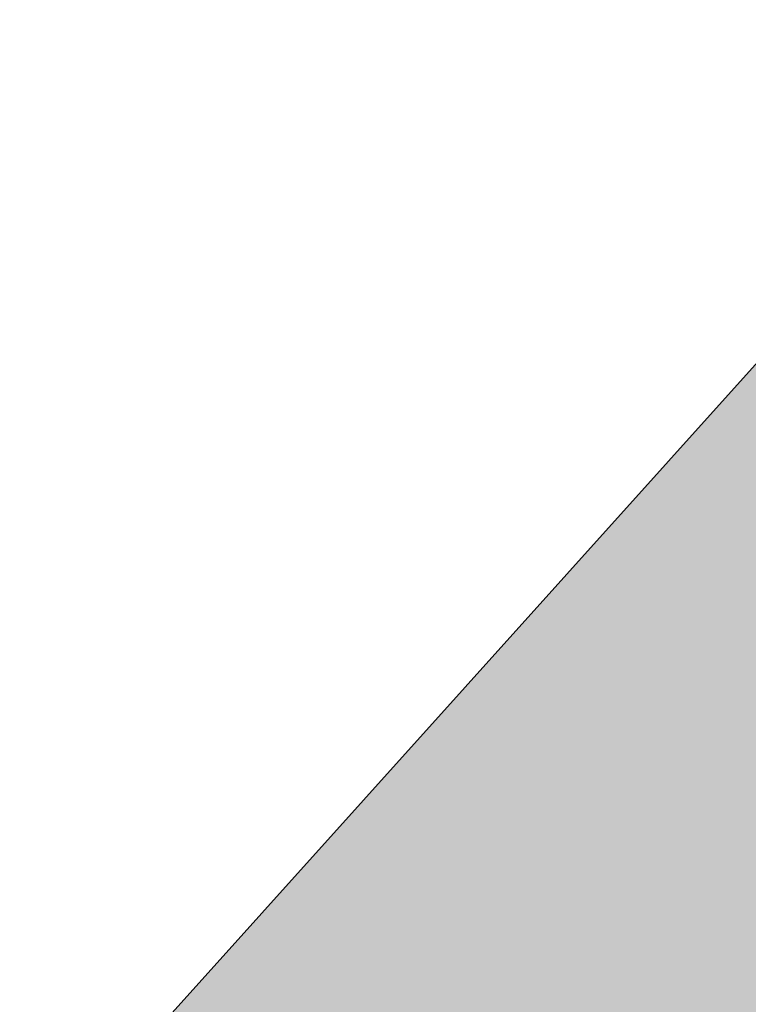
# Model space of a CAD drawing. Units: inches. Extents: x 2091 to 2899, y 967 to 2217.
# Tile 246 of 256: x 2213.354327 to 2213.360613, y 1136.678717 to 1136.687206. Entities that reach past the tile are written whole.
import ezdxf

# ---------------------------------------------------------------- set-up
doc = ezdxf.new("R2010")
doc.units = ezdxf.units.IN
doc.layers.add('L-PLNT-PATT', color=114, linetype='Continuous', lineweight=13, true_color=0x139b48)
doc.layers.add('L-PLNT-TREE', color=94, linetype='Continuous', lineweight=13)

# ---------------------------------------------------------------- blocks, each defined once
blk = doc.blocks.new('*U25')
blk.add_lwpolyline([(-1139.42368, 1783.79628), (-1216.11644, 1685.47796), (-1117.5111, 1601.2033), (-1051.7759, 1643.3419), (-1126.09884, 1521.20092), (-1072.10606, 1527.49758), (-1079.90386, 1416.93646), (-1259.93906, 1179.83508), (-1479.05978, 1165.78888), (-1577.66258, 1109.60662), (-1742.00312, 927.01364), (-1676.26538, 814.64658), (-1270.89408, 828.69278), (-1194.20386, 772.51052), (-1007.95074, 856.78518), (-876.4778, 575.87134), (-821.70016, 575.87134), (-569.71184, 884.87504)])

msp = doc.modelspace()

# ---------------------------------------------------------------- hatches: boundary and pattern name
at = {"layer": 'L-PLNT-PATT'}
h = msp.add_hatch(color=256, dxfattribs=at)
h.dxf.hatch_style = 1
h.paths.add_polyline_path([(2333.3376413, 1165.6587034), (2329.0242413, 1166.2116034), (2331.6122413, 1168.4235034), (2335.0629413, 1177.2712034), (2328.1615413, 1184.4599034), (2319.5348413, 1187.2248034), (2323.4168413, 1193.3076034), (2319.9661413, 1203.8142034), (2317.8094413, 1203.8142034), (2313.4960413, 1213.2148034), (2310.9080413, 1212.6618034), (2307.8887413, 1212.6618034), (2305.7319413, 1217.0857034), (2307.0259413, 1223.1684034), (2310.4767413, 1223.1684034), (2304.0066413, 1230.9101034), (2303.1363444, 1237.0464689), (2299.6932413, 1240.8637034), (2296.6739413, 1237.5459034), (2294.9485413, 1238.6518034), (2294.5171413, 1241.4166034), (2292.3605413, 1242.5227034), (2289.3411413, 1239.7577034), (2285.8904413, 1240.3107034), (2283.3024413, 1235.3339034), (2283.3024413, 1230.9101034), (2286.7531413, 1229.2512034), (2284.1650413, 1227.5922034), (2281.5770413, 1229.8042034), (2274.2442413, 1222.6154034), (2274.2442413, 1220.9565034), (2271.2249413, 1219.2976034), (2272.0876413, 1217.6386034), (2274.2442413, 1214.3208034), (2270.3622413, 1211.5559034), (2266.4801413, 1214.3208034), (2264.3235413, 1213.7678034), (2263.4608413, 1211.5559034), (2266.4801413, 1211.0029034), (2266.9115413, 1206.5791034), (2263.5392413, 1207.1320034), (2259.5788413, 1203.2612034), (2263.8921413, 1202.7082034), (2262.1668413, 1197.1784034), (2258.2848413, 1196.6254034), (2253.9714413, 1193.8606034), (2248.7953413, 1191.0957034), (2248.3640413, 1193.3076034), (2244.4819413, 1185.0129034), (2251.3833413, 1186.6718034), (2255.6967413, 1183.9069034), (2254.4027413, 1177.2712034), (2246.6387413, 1174.5063034), (2243.1879413, 1176.7182034), (2241.8939413, 1173.4003034), (2238.8746413, 1172.8474034), (2236.2865413, 1169.5295034), (2233.2671413, 1165.6587034), (2237.1492413, 1162.3408034), (2239.7372413, 1163.9998034), (2236.8111413, 1159.1911034), (2238.9368413, 1159.4390034), (2238.6298413, 1155.0862034), (2231.5418413, 1145.7515034), (2222.9150413, 1145.1985034), (2219.0330413, 1142.9866034), (2212.5629413, 1135.7979034), (2215.1510413, 1131.3740034), (2231.1105413, 1131.9270034), (2234.1298413, 1129.7151034), (2241.4626413, 1133.0330034), (2246.6387413, 1121.9734034), (2248.7953413, 1121.9734034), (2258.7161413, 1134.1389034), (2261.7355413, 1135.7979034), (2263.8921413, 1133.0330034), (2263.8921413, 1129.1621034), (2267.3429413, 1128.0562034), (2272.0876413, 1128.0562034), (2273.8129413, 1131.9270034), (2279.4203413, 1134.6919034), (2285.0278413, 1135.2449034), (2287.6158413, 1137.4568034), (2288.0471413, 1138.0098034), (2289.3411413, 1140.7747034), (2291.0665413, 1139.6687034), (2292.3605413, 1135.2449034), (2295.3798413, 1136.9038034), (2296.2425413, 1135.7979034), (2297.1052413, 1133.0330034), (2300.1246413, 1138.0098034), (2303.1439413, 1138.0098034), (2304.4379413, 1135.7979034), (2303.1439413, 1133.5860034), (2306.5946413, 1134.6919034), (2307.8887413, 1133.0330034), (2310.9080413, 1135.2449034), (2313.9274413, 1134.1389034), (2319.9661413, 1128.0562034), (2322.5541413, 1126.9502034), (2324.7108413, 1124.7383034), (2342.8270413, 1126.3972034), (2346.2777413, 1123.0794034), (2348.8658413, 1124.1853034), (2341.9643413, 1133.0330034), (2341.5330413, 1136.3508034), (2343.6897413, 1139.6687034), (2339.8077413, 1150.1753034), (2337.6510413, 1150.1753034)])
h.paths.add_polyline_path([(2339.6577999, 1120.6164204), (2337.9037999, 1120.3574204), (2338.4437999, 1119.5784204), (2340.3327999, 1119.6654204)])
h.paths.add_polyline_path([(2341.1427999, 1118.5404204), (2339.0507999, 1118.6264204), (2339.0507999, 1117.6754204), (2340.9407999, 1116.9824204)])
h.paths.add_polyline_path([(2336.5537999, 1120.8764204), (2335.2037999, 1120.3574204), (2334.7987999, 1118.9724204), (2336.8237999, 1119.5784204)])
h.paths.add_polyline_path([(2337.2957999, 1118.9724204), (2336.6207999, 1118.2804204), (2337.6337999, 1117.7614204)])
h.paths.add_polyline_path([(2338.6457999, 1118.7134204), (2339.1857999, 1119.3194204), (2338.2407999, 1118.8864204), (2338.2407999, 1118.1074204)])
h.paths.add_polyline_path([(2339.0507999, 1122.8664204), (2337.7687999, 1123.8184204), (2337.0937999, 1123.1254204), (2337.2957999, 1121.8284204)])
h.paths.add_polyline_path([(2341.6147999, 1122.0014204), (2341.1427999, 1121.8284204), (2340.6707999, 1122.9524204), (2340.1307999, 1121.8284204), (2340.5357999, 1121.0494204), (2341.7497999, 1120.5304204), (2342.8297999, 1121.2224204)])
h.paths.add_polyline_path([(2342.9647999, 1119.7514204), (2342.0197999, 1119.4914204), (2342.0877999, 1118.0214204), (2343.0327999, 1118.4534204)])
h.paths.add_polyline_path([(2345.8667999, 1118.1944204), (2344.3827999, 1118.6264204), (2343.7077999, 1118.0214204), (2345.5297999, 1117.3294204)])
h.paths.add_polyline_path([(2344.6517999, 1116.8094204), (2343.6397999, 1116.4634204), (2343.0327999, 1115.9444204), (2343.9097999, 1114.9064204), (2344.6517999, 1115.3394204), (2344.1797999, 1115.6854204)])
h.paths.add_polyline_path([(2346.8117999, 1116.9824204), (2345.7317999, 1115.8584204), (2345.5297999, 1114.1274204), (2347.0137999, 1112.3104204), (2348.2967999, 1112.2244204), (2346.8797999, 1114.3004204), (2345.8667999, 1114.2144204), (2346.8117999, 1114.6464204)])
h.paths.add_polyline_path([(2345.2597999, 1116.5504204), (2344.7197999, 1116.3774204), (2344.9217999, 1115.6854204), (2345.1247999, 1115.8584204)])
h.paths.add_polyline_path([(2342.6947999, 1116.8964204), (2342.0197999, 1117.3294204), (2341.9527999, 1116.6364204)])
h.paths.add_polyline_path([(2341.4807999, 1120.0974204), (2341.1427999, 1120.0974204), (2341.0757999, 1119.5784204), (2341.4807999, 1119.4054204)])
h.paths.add_polyline_path([(2343.9777999, 1121.1354204), (2343.6397999, 1119.7514204), (2345.0567999, 1119.7514204)])
h.paths.add_polyline_path([(2339.1177999, 1121.7414204), (2338.3757999, 1121.5684204), (2338.1737999, 1121.0494204), (2338.8477999, 1121.2224204)])
h.paths.add_polyline_path([(2336.3507999, 1122.4334204), (2335.7437999, 1122.7794204), (2334.5287999, 1123.4714204), (2334.9337999, 1122.4334204), (2336.0137999, 1121.9144204)])
h.paths.add_polyline_path([(2334.4617999, 1122.1744204), (2332.0997999, 1122.8664204), (2331.3567999, 1122.1744204), (2332.5717999, 1121.3084204)])
h.paths.add_polyline_path([(2334.5967999, 1121.3084204), (2334.0567999, 1120.7894204), (2334.2587999, 1120.3574204), (2334.7317999, 1120.8764204)])
h.paths.add_polyline_path([(2332.5047999, 1120.7894204), (2331.6947999, 1120.4434204), (2332.7067999, 1119.6654204)])
h.paths.add_polyline_path([(2333.6517999, 1119.3194204), (2333.3817999, 1118.4534204), (2334.2587999, 1118.5404204)])
h.paths.add_polyline_path([(2331.9647999, 1118.1944204), (2331.0867999, 1116.2904204), (2332.6397999, 1116.6364204)])
h.paths.add_polyline_path([(2330.7497999, 1121.5684204), (2328.9947999, 1121.0494204), (2328.5227999, 1119.3194204), (2330.2767999, 1120.2704204)])
h.paths.add_polyline_path([(2330.7497999, 1118.6264204), (2329.8727999, 1118.0214204), (2330.0077999, 1117.5024204)])
h.paths.add_polyline_path([(2328.3877999, 1117.8484204), (2327.1727999, 1117.7614204), (2327.5097999, 1116.5504204)])
h.paths.add_polyline_path([(2326.9027999, 1115.2524204), (2326.0927999, 1115.3394204), (2325.2157999, 1113.6084204), (2326.7007999, 1114.1274204)])
h.paths.add_polyline_path([(2328.6577999, 1114.3874204), (2328.3197999, 1114.9064204), (2328.0497999, 1114.1274204)])
h.paths.add_polyline_path([(2326.7007999, 1112.6564204), (2327.1057999, 1112.1374204), (2328.3197999, 1112.2244204)])
h.paths.add_polyline_path([(2329.5347999, 1113.6084204), (2328.5897999, 1113.3494204), (2329.0627999, 1112.3104204)])
h.paths.add_polyline_path([(2340.3327999, 1115.3394204), (2339.3877999, 1115.3394204), (2340.0627999, 1113.6954204)])
h.paths.add_polyline_path([(2340.9407999, 1116.3774204), (2340.8057999, 1115.5124204), (2342.0197999, 1115.0794204)])
h.paths.add_polyline_path([(2341.8177999, 1114.4734204), (2340.8057999, 1114.5604204), (2340.9407999, 1113.0894204)])
h.paths.add_polyline_path([(2343.0327999, 1112.2244204), (2342.3577999, 1113.3494204), (2341.5477999, 1112.2244204), (2342.0197999, 1111.7914204)])
h.paths.add_polyline_path([(2342.7627999, 1113.9544204), (2343.4377999, 1113.0894204), (2344.0447999, 1113.5224204)])
h.paths.add_polyline_path([(2344.7197999, 1114.3874204), (2344.4497999, 1113.8684204), (2345.1917999, 1113.3494204)])
h.paths.add_polyline_path([(2345.6647999, 1112.3104204), (2344.6517999, 1112.5704204), (2344.0447999, 1111.9644204), (2345.4617999, 1111.5324204)])
h.paths.add_polyline_path([(2344.3147999, 1111.0124204), (2342.9647999, 1111.0994204), (2342.9647999, 1110.3204204)])
h.paths.add_polyline_path([(2344.8547999, 1110.0614204), (2344.1127999, 1109.7154204), (2344.5167999, 1109.2824204)])
h.paths.add_polyline_path([(2346.6767999, 1109.2824204), (2345.8667999, 1110.0614204), (2346.0697999, 1108.0714204)])
h.paths.add_polyline_path([(2347.0137999, 1110.9264204), (2346.6097999, 1111.1864204), (2346.2717999, 1110.4934204)])
h.paths.add_polyline_path([(2345.8667999, 1106.6864204), (2344.5167999, 1106.6004204), (2344.9897999, 1105.5624204)])
h.paths.add_polyline_path([(2345.1247999, 1104.6974204), (2344.4497999, 1104.2644204), (2344.5847999, 1103.7454204)])
h.paths.add_polyline_path([(2343.7747999, 1104.4374204), (2343.4377999, 1105.1294204), (2342.6947999, 1104.6104204), (2342.6277999, 1102.8804204)])
h.paths.add_polyline_path([(2341.8177999, 1103.8314204), (2341.1427999, 1103.6584204), (2341.5477999, 1102.8804204)])
h.paths.add_polyline_path([(2342.5597999, 1102.3614204), (2341.9527999, 1101.8414204), (2342.6947999, 1101.6684204)])
h.paths.add_polyline_path([(2341.1427999, 1101.9284204), (2340.6027999, 1102.3614204), (2340.0627999, 1101.8414204), (2340.6027999, 1101.2364204)])
h.paths.add_polyline_path([(2336.7557999, 1101.2364204), (2337.3637999, 1100.5434204), (2339.1177999, 1100.4574204)])
h.paths.add_polyline_path([(2335.2717999, 1103.3124204), (2334.1917999, 1102.6204204), (2335.5417999, 1102.2744204)])
h.paths.add_polyline_path([(2333.9887999, 1101.7554204), (2333.5167999, 1101.5824204), (2334.7317999, 1101.1494204)])
h.paths.add_polyline_path([(2331.6947999, 1102.9664204), (2330.5467999, 1102.0144204), (2332.0997999, 1102.3614204)])
h.paths.add_polyline_path([(2329.7377999, 1106.5134204), (2328.2527999, 1106.0814204), (2329.5347999, 1105.3024204)])
h.paths.add_polyline_path([(2326.6327999, 1108.3304204), (2326.4977999, 1109.1094204), (2325.8907999, 1108.5034204), (2326.0927999, 1107.3794204)])
h.paths.add_polyline_path([(2240.5960787, 1257.814216), (2239.5840787, 1257.468216), (2238.9770787, 1256.949216), (2239.8540787, 1255.911216), (2240.5960787, 1256.344216), (2240.1240787, 1256.690216)])
h.paths.add_polyline_path([(2241.8110787, 1259.199216), (2240.3270787, 1259.631216), (2239.6520787, 1259.026216), (2241.4740787, 1258.334216)])
h.paths.add_polyline_path([(2242.7560787, 1257.987216), (2241.6760787, 1256.863216), (2241.4740787, 1255.132216), (2242.9580787, 1253.315216), (2244.2410787, 1253.229216), (2242.8240787, 1255.305216), (2241.8110787, 1255.219216), (2242.7560787, 1255.651216)])
h.paths.add_polyline_path([(2241.6090787, 1253.315216), (2240.5960787, 1253.575216), (2239.9890787, 1252.969216), (2241.4060787, 1252.537216)])
h.paths.add_polyline_path([(2240.6640787, 1255.392216), (2240.3940787, 1254.873216), (2241.1360787, 1254.354216)])
h.paths.add_polyline_path([(2242.9580787, 1251.931216), (2242.5540787, 1252.191216), (2242.2160787, 1251.498216)])
h.paths.add_polyline_path([(2240.2590787, 1252.017216), (2238.9090787, 1252.104216), (2238.9090787, 1251.325216)])
h.paths.add_polyline_path([(2238.3020787, 1254.354216), (2237.4920787, 1253.229216), (2237.9640787, 1252.796216), (2238.9770787, 1253.229216)])
h.paths.add_polyline_path([(2239.9890787, 1254.527216), (2238.7070787, 1254.959216), (2239.3820787, 1254.094216)])
h.paths.add_polyline_path([(2240.7990787, 1251.066216), (2240.0570787, 1250.720216), (2240.4610787, 1250.287216)])
h.paths.add_polyline_path([(2241.8110787, 1251.066216), (2242.0140787, 1249.076216), (2242.6210787, 1250.287216)])
h.paths.add_polyline_path([(2241.2040787, 1257.555216), (2240.6640787, 1257.382216), (2240.8660787, 1256.690216), (2241.0690787, 1256.863216)])
h.paths.add_polyline_path([(2238.6390787, 1257.901216), (2237.9640787, 1258.334216), (2237.8970787, 1257.641216)])
h.paths.add_polyline_path([(2238.9090787, 1260.756216), (2237.9640787, 1260.496216), (2238.0320787, 1259.026216), (2238.9770787, 1259.458216)])
h.paths.add_polyline_path([(2239.9220787, 1262.140216), (2239.5840787, 1260.756216), (2241.0010787, 1260.756216)])
h.paths.add_polyline_path([(2238.7740787, 1262.227216), (2237.5590787, 1263.006216), (2237.0870787, 1262.833216), (2236.6150787, 1263.957216), (2236.0750787, 1262.833216), (2236.4800787, 1262.054216), (2237.6940787, 1261.535216)])
h.paths.add_polyline_path([(2237.4250787, 1261.102216), (2237.0870787, 1261.102216), (2237.0200787, 1260.583216), (2237.4250787, 1260.410216)])
h.paths.add_polyline_path([(2237.0870787, 1259.545216), (2234.9950787, 1259.631216), (2234.9950787, 1258.680216), (2236.8850787, 1257.987216)])
h.paths.add_polyline_path([(2236.8850787, 1257.382216), (2236.7500787, 1256.517216), (2237.9640787, 1256.084216)])
h.paths.add_polyline_path([(2237.7620787, 1255.478216), (2236.7500787, 1255.565216), (2236.8850787, 1254.094216)])
h.paths.add_polyline_path([(2236.2770787, 1256.344216), (2235.3320787, 1256.344216), (2236.0070787, 1254.700216)])
h.paths.add_polyline_path([(2241.8110787, 1247.691216), (2240.4610787, 1247.605216), (2240.9340787, 1246.567216)])
h.paths.add_polyline_path([(2239.7190787, 1245.442216), (2239.3820787, 1246.134216), (2238.6390787, 1245.615216), (2238.5720787, 1243.885216)])
h.paths.add_polyline_path([(2241.0690787, 1245.702216), (2240.3940787, 1245.269216), (2240.5290787, 1244.750216)])
h.paths.add_polyline_path([(2237.7620787, 1244.836216), (2237.0870787, 1244.663216), (2237.4920787, 1243.885216)])
h.paths.add_polyline_path([(2237.0870787, 1242.933216), (2236.5470787, 1243.366216), (2236.0070787, 1242.846216), (2236.5470787, 1242.241216)])
h.paths.add_polyline_path([(2238.5040787, 1243.366216), (2237.8970787, 1242.846216), (2238.6390787, 1242.673216)])
h.paths.add_polyline_path([(2232.7000787, 1242.241216), (2233.3080787, 1241.548216), (2235.0620787, 1241.462216)], flags=17)
h.paths.add_polyline_path([(2231.2160787, 1244.317216), (2230.1360787, 1243.625216), (2231.4860787, 1243.279216)])
h.paths.add_polyline_path([(2229.9330787, 1242.760216), (2229.4610787, 1242.587216), (2230.6760787, 1242.154216)])
h.paths.add_polyline_path([(2227.6390787, 1243.971216), (2226.4910787, 1243.019216), (2228.0440787, 1243.366216)])
h.paths.add_polyline_path([(2222.5770787, 1249.335216), (2222.4420787, 1250.114216), (2221.8350787, 1249.508216), (2222.0370787, 1248.384216)])
h.paths.add_polyline_path([(2225.6820787, 1247.518216), (2224.1970787, 1247.086216), (2225.4790787, 1246.307216)])
h.paths.add_polyline_path([(2225.4790787, 1254.613216), (2224.5340787, 1254.354216), (2225.0070787, 1253.315216)])
h.paths.add_polyline_path([(2224.2640787, 1253.229216), (2222.6450787, 1253.661216), (2223.0500787, 1253.142216)])
h.paths.add_polyline_path([(2222.8470787, 1256.257216), (2222.0370787, 1256.344216), (2221.1600787, 1254.613216), (2222.6450787, 1255.132216)])
h.paths.add_polyline_path([(2224.3320787, 1258.853216), (2223.1170787, 1258.766216), (2223.4540787, 1257.555216)])
h.paths.add_polyline_path([(2226.6940787, 1259.631216), (2225.8170787, 1259.026216), (2225.9520787, 1258.507216)])
h.paths.add_polyline_path([(2227.9090787, 1259.199216), (2227.0310787, 1257.295216), (2228.5840787, 1257.641216)])
h.paths.add_polyline_path([(2224.2640787, 1255.911216), (2223.9940787, 1255.132216), (2224.6020787, 1255.392216)])
h.paths.add_polyline_path([(2229.5960787, 1260.324216), (2229.3260787, 1259.458216), (2230.2030787, 1259.545216)])
h.paths.add_polyline_path([(2228.4490787, 1261.794216), (2227.6390787, 1261.448216), (2228.6510787, 1260.670216)])
h.paths.add_polyline_path([(2230.4060787, 1263.179216), (2228.0440787, 1263.871216), (2227.3010787, 1263.179216), (2228.5160787, 1262.313216)])
h.paths.add_polyline_path([(2232.7680787, 1260.583216), (2232.4980787, 1261.881216), (2231.1480787, 1261.362216), (2230.7430787, 1259.977216)])
h.paths.add_polyline_path([(2230.6760787, 1261.881216), (2230.5410787, 1262.313216), (2230.0010787, 1261.794216), (2230.2030787, 1261.362216)])
h.paths.add_polyline_path([(2232.2950787, 1263.438216), (2231.6880787, 1263.784216), (2230.4730787, 1264.476216), (2230.8780787, 1263.438216), (2231.9580787, 1262.919216)])
h.paths.add_polyline_path([(2234.9950787, 1263.871216), (2233.7130787, 1264.823216), (2233.0380787, 1264.130216), (2233.2400787, 1262.833216)])
h.paths.add_polyline_path([(2235.0620787, 1262.746216), (2234.3200787, 1262.573216), (2234.1180787, 1262.054216), (2234.7920787, 1262.227216)])
h.paths.add_polyline_path([(2235.6020787, 1261.621216), (2233.8480787, 1261.362216), (2234.3880787, 1260.583216), (2236.2770787, 1260.670216)])
h.paths.add_polyline_path([(2235.1300787, 1260.324216), (2234.1850787, 1259.891216), (2234.1850787, 1259.112216), (2234.5900787, 1259.718216)])
h.paths.add_polyline_path([(2226.6940787, 1262.573216), (2224.9390787, 1262.054216), (2224.4670787, 1260.324216), (2226.2210787, 1261.275216)])
h.paths.add_polyline_path([(2233.2400787, 1259.977216), (2232.5650787, 1259.285216), (2233.5780787, 1258.766216)])
h.paths.add_polyline_path([(2337.2674406, 1337.8274829), (2336.1874406, 1336.7034829), (2335.9854406, 1334.9724829), (2337.4694406, 1333.1554829), (2338.7524406, 1333.0694829), (2337.3354406, 1335.1454829), (2336.3224406, 1335.0594829), (2337.2674406, 1335.4914829)])
h.paths.add_polyline_path([(2336.3224406, 1339.0394829), (2334.8384406, 1339.4714829), (2334.1634406, 1338.8664829), (2335.9854406, 1338.1744829)])
h.paths.add_polyline_path([(2334.4334406, 1341.9804829), (2334.0954406, 1340.5964829), (2335.5124406, 1340.5964829)])
h.paths.add_polyline_path([(2333.2854406, 1342.0674829), (2332.0704406, 1342.8464829), (2331.5984406, 1342.6734829), (2331.1264406, 1343.7974829), (2330.5864406, 1342.6734829), (2330.9914406, 1341.8944829), (2332.2054406, 1341.3754829)])
h.paths.add_polyline_path([(2333.4204406, 1340.5964829), (2332.4754406, 1340.3364829), (2332.5434406, 1338.8664829), (2333.4884406, 1339.2984829)])
h.paths.add_polyline_path([(2331.9364406, 1340.9424829), (2331.5984406, 1340.9424829), (2331.5314406, 1340.4234829), (2331.9364406, 1340.2504829)])
h.paths.add_polyline_path([(2329.5734406, 1342.5864829), (2328.8314406, 1342.4134829), (2328.6294406, 1341.8944829), (2329.3034406, 1342.0674829)])
h.paths.add_polyline_path([(2329.5064406, 1343.7114829), (2328.2244406, 1344.6634829), (2327.5494406, 1343.9704829), (2327.7514406, 1342.6734829)])
h.paths.add_polyline_path([(2330.1134406, 1341.4614829), (2328.3594406, 1341.2024829), (2328.8994406, 1340.4234829), (2330.7884406, 1340.5104829)])
h.paths.add_polyline_path([(2331.5984406, 1339.3854829), (2329.5064406, 1339.4714829), (2329.5064406, 1338.5204829), (2331.3964406, 1337.8274829)])
h.paths.add_polyline_path([(2327.0094406, 1341.7214829), (2325.6594406, 1341.2024829), (2325.2544406, 1339.8174829), (2327.2794406, 1340.4234829)])
h.paths.add_polyline_path([(2326.8064406, 1343.2784829), (2326.1994406, 1343.6244829), (2324.9844406, 1344.3164829), (2325.3894406, 1343.2784829), (2326.4694406, 1342.7594829)])
h.paths.add_polyline_path([(2324.9174406, 1343.0194829), (2322.5554406, 1343.7114829), (2321.8124406, 1343.0194829), (2323.0274406, 1342.1534829)])
h.paths.add_polyline_path([(2321.2054406, 1342.4134829), (2319.4504406, 1341.8944829), (2318.9784406, 1340.1644829), (2320.7324406, 1341.1154829)])
h.paths.add_polyline_path([(2318.8434406, 1338.6934829), (2317.6284406, 1338.6064829), (2317.9654406, 1337.3954829)])
h.paths.add_polyline_path([(2322.4204406, 1339.0394829), (2321.5424406, 1337.1354829), (2323.0954406, 1337.4814829)])
h.paths.add_polyline_path([(2324.1074406, 1340.1644829), (2323.8374406, 1339.2984829), (2324.7144406, 1339.3854829)])
h.paths.add_polyline_path([(2322.9604406, 1341.6344829), (2322.1504406, 1341.2884829), (2323.1624406, 1340.5104829)])
h.paths.add_polyline_path([(2325.1874406, 1341.7214829), (2325.0524406, 1342.1534829), (2324.5124406, 1341.6344829), (2324.7144406, 1341.2024829)])
h.paths.add_polyline_path([(2321.2054406, 1339.4714829), (2320.3284406, 1338.8664829), (2320.4634406, 1338.3474829)])
h.paths.add_polyline_path([(2317.3584406, 1336.0974829), (2316.5484406, 1336.1844829), (2315.6714406, 1334.4534829), (2317.1564406, 1334.9724829)])
h.paths.add_polyline_path([(2318.7754406, 1335.7514829), (2318.5054406, 1334.9724829), (2319.1134406, 1335.2324829)])
h.paths.add_polyline_path([(2319.9904406, 1334.4534829), (2319.0454406, 1334.1944829), (2319.5184406, 1333.1554829)])
h.paths.add_polyline_path([(2317.1564406, 1333.5014829), (2317.5614406, 1332.9824829), (2318.7754406, 1333.0694829)])
h.paths.add_polyline_path([(2317.0884406, 1329.1754829), (2316.9534406, 1329.9544829), (2316.3464406, 1329.3484829), (2316.5484406, 1328.2244829)])
h.paths.add_polyline_path([(2320.1934406, 1327.3584829), (2318.7084406, 1326.9264829), (2319.9904406, 1326.1474829)])
h.paths.add_polyline_path([(2322.1504406, 1323.8114829), (2321.0024406, 1322.8594829), (2322.5554406, 1323.2064829)])
h.paths.add_polyline_path([(2325.7274406, 1324.1574829), (2324.6474406, 1323.4654829), (2325.9974406, 1323.1194829)])
h.paths.add_polyline_path([(2334.2304406, 1325.2824829), (2333.8934406, 1325.9744829), (2333.1504406, 1325.4554829), (2333.0834406, 1323.7254829)])
h.paths.add_polyline_path([(2336.3224406, 1327.5314829), (2334.9724406, 1327.4454829), (2335.4454406, 1326.4074829)])
h.paths.add_polyline_path([(2335.3104406, 1330.9064829), (2334.5684406, 1330.5604829), (2334.9724406, 1330.1274829)])
h.paths.add_polyline_path([(2334.7704406, 1331.8574829), (2333.4204406, 1331.9444829), (2333.4204406, 1331.1654829)])
h.paths.add_polyline_path([(2332.8134406, 1334.1944829), (2332.0034406, 1333.0694829), (2332.4754406, 1332.6364829), (2333.4884406, 1333.0694829)])
h.paths.add_polyline_path([(2335.1074406, 1333.4154829), (2334.5004406, 1332.8094829), (2335.9174406, 1332.3774829), (2336.1204406, 1333.1554829)])
h.paths.add_polyline_path([(2334.6354406, 1336.5304829), (2335.1074406, 1337.6544829), (2334.0954406, 1337.3084829), (2333.4884406, 1336.7894829), (2334.3654406, 1335.7514829), (2335.1074406, 1336.1844829)])
h.paths.add_polyline_path([(2335.7154406, 1337.3954829), (2335.1754406, 1337.2224829), (2335.3774406, 1336.5304829), (2335.5804406, 1336.7034829)])
h.paths.add_polyline_path([(2333.1504406, 1337.7414829), (2332.4754406, 1338.1744829), (2332.4084406, 1337.4814829)])
h.paths.add_polyline_path([(2330.7884406, 1336.1844829), (2329.8434406, 1336.1844829), (2330.5184406, 1334.5404829)])
h.paths.add_polyline_path([(2332.2734406, 1335.3184829), (2331.2614406, 1335.4054829), (2331.3964406, 1333.9344829)])
h.paths.add_polyline_path([(2331.3964406, 1337.2224829), (2331.2614406, 1336.3574829), (2332.4754406, 1335.9244829)])
h.paths.add_polyline_path([(2334.5004406, 1334.3674829), (2333.2184406, 1334.7994829), (2333.8934406, 1333.9344829)])
h.paths.add_polyline_path([(2335.1754406, 1335.2324829), (2334.9054406, 1334.7134829), (2335.6474406, 1334.1944829)])
h.paths.add_polyline_path([(2337.1324406, 1330.1274829), (2336.3224406, 1330.9064829), (2336.5254406, 1328.9164829)])
h.paths.add_polyline_path([(2337.0654406, 1332.0314829), (2336.7274406, 1331.3384829), (2337.4694406, 1331.7714829)])
h.paths.add_polyline_path([(2329.6414406, 1340.1644829), (2328.6964406, 1339.7314829), (2328.6964406, 1338.9524829), (2329.1014406, 1339.5584829)])
h.paths.add_polyline_path([(2327.7514406, 1339.8174829), (2327.0764406, 1339.1254829), (2328.0894406, 1338.6064829)])
h.paths.add_polyline_path([(2327.2114406, 1322.0814829), (2327.8194406, 1321.3884829), (2329.5734406, 1321.3024829)])
h.paths.add_polyline_path([(2324.4444406, 1322.6004829), (2323.9724406, 1322.4274829), (2325.1874406, 1321.9944829)])
h.paths.add_polyline_path([(2331.0584406, 1323.2064829), (2330.5184406, 1322.6864829), (2331.0584406, 1322.0814829), (2331.5984406, 1322.7734829)])
h.paths.add_polyline_path([(2332.2734406, 1324.6764829), (2331.5984406, 1324.5034829), (2332.0034406, 1323.7254829)])
h.paths.add_polyline_path([(2333.0154406, 1323.2064829), (2332.4084406, 1322.6864829), (2333.1504406, 1322.5134829)])
h.paths.add_polyline_path([(2335.5804406, 1325.5424829), (2334.9054406, 1325.1094829), (2335.0404406, 1324.5904829)])
h.paths.add_polyline_path([(2271.0827276, 1964.3172377), (2776.852968, 1964.3172377), (2776.852968, 2037.1696226), (2271.0827276, 2037.1696226)], flags=9)
h.paths.add_polyline_path([(2380.6492852, 1536.8241435), (2461.0408087, 1536.8241435), (2461.0408087, 1554.6525871), (2380.6492852, 1554.6525871)], flags=9)
h.paths.add_polyline_path([(2240.7557092, 1609.7254508), (2309.1858294, 1609.7254508), (2309.1858294, 1617.6982037), (2240.7557092, 1617.6982037)], flags=9)
h.paths.add_polyline_path([(2212.6772554, 1313.5041021), (2282.5915203, 1313.5041021), (2282.5915203, 1322.7452389), (2212.6772554, 1322.7452389)], flags=9)
h.paths.add_polyline_path([(2457.111976, 1114.778574), (2558.4815807, 1114.778574), (2558.4815807, 1142.2196823), (2457.111976, 1142.2196823)], flags=9)
h.paths.add_polyline_path([(2473.4423372, 1273.0100672), (2604.6412257, 1273.0100672), (2604.6412257, 1318.3469349), (2473.4423372, 1318.3469349)], flags=9)
h.paths.add_polyline_path([(2638.8763024, 1626.9774316), (2684.2503675, 1627.9767377), (2684.0384825, 1637.5974944), (2638.6644174, 1636.5981884)], flags=9)
h.paths.add_polyline_path([(2537.5905538, 1453.7934466), (2628.3895472, 1453.7934466), (2628.3895472, 1475.3448114), (2537.5905538, 1475.3448114)], flags=9)
h.paths.add_polyline_path([(2504.1376376, 1714.6323972), (2554.6471875, 1714.6323972), (2554.6471875, 1730.2377115), (2504.1376376, 1730.2377115)], flags=9)
h.paths.add_polyline_path([(2487.5011806, 1575.6518716), (2535.0971214, 1575.6518716), (2535.0971214, 1598.3776456), (2487.5011806, 1598.3776456)], flags=9)
h.paths.add_polyline_path([(2709.0994004, 1735.7102784), (2740.0166009, 1735.7102784), (2740.0166009, 1749.9376406), (2709.0994004, 1749.9376406)], flags=9)
h.paths.add_polyline_path([(2442.4384239, 1792.1716575), (2564.7288353, 1792.1716575), (2564.7288353, 1842.0001626), (2442.4384239, 1842.0001626)], flags=9)
h.paths.add_polyline_path([(2655.8158012, 1809.6440763), (2789.5201425, 1806.6937963), (2790.0849768, 1832.2916379), (2656.3806355, 1835.2419179)], flags=9)
h.paths.add_polyline_path([(2234.8426972, 1797.7201432), (2368.5928512, 1794.7688523), (2369.1607182, 1820.504132), (2235.4105642, 1823.4554229)], flags=9)
h.paths.add_polyline_path([(2245.1384659, 1644.0063348), (2398.4277329, 1640.6238997), (2398.9948417, 1666.3248199), (2245.7055747, 1669.7072549)], flags=9)
h.paths.add_polyline_path([(2306.1428474, 1431.1685186), (2413.7683138, 1428.7936873), (2414.3331481, 1454.3915289), (2306.7076817, 1456.7663602)], flags=9)
h.paths.add_polyline_path([(2306.834582, 1458.2331447), (2393.3804836, 1456.3234487), (2393.9328082, 1481.3543583), (2307.3869066, 1483.2640542)], flags=9)

# ---------------------------------------------------------------- block references
at = {"layer": 'L-PLNT-TREE', "xscale": 0.0393700787401575, "yscale": 0.0393700787401575, "zscale": 0.0393700787401575}
msp.add_blockref('*U25', (2281.1457413, 1099.3013034), dxfattribs=at)

doc.saveas('drawing.dxf')
